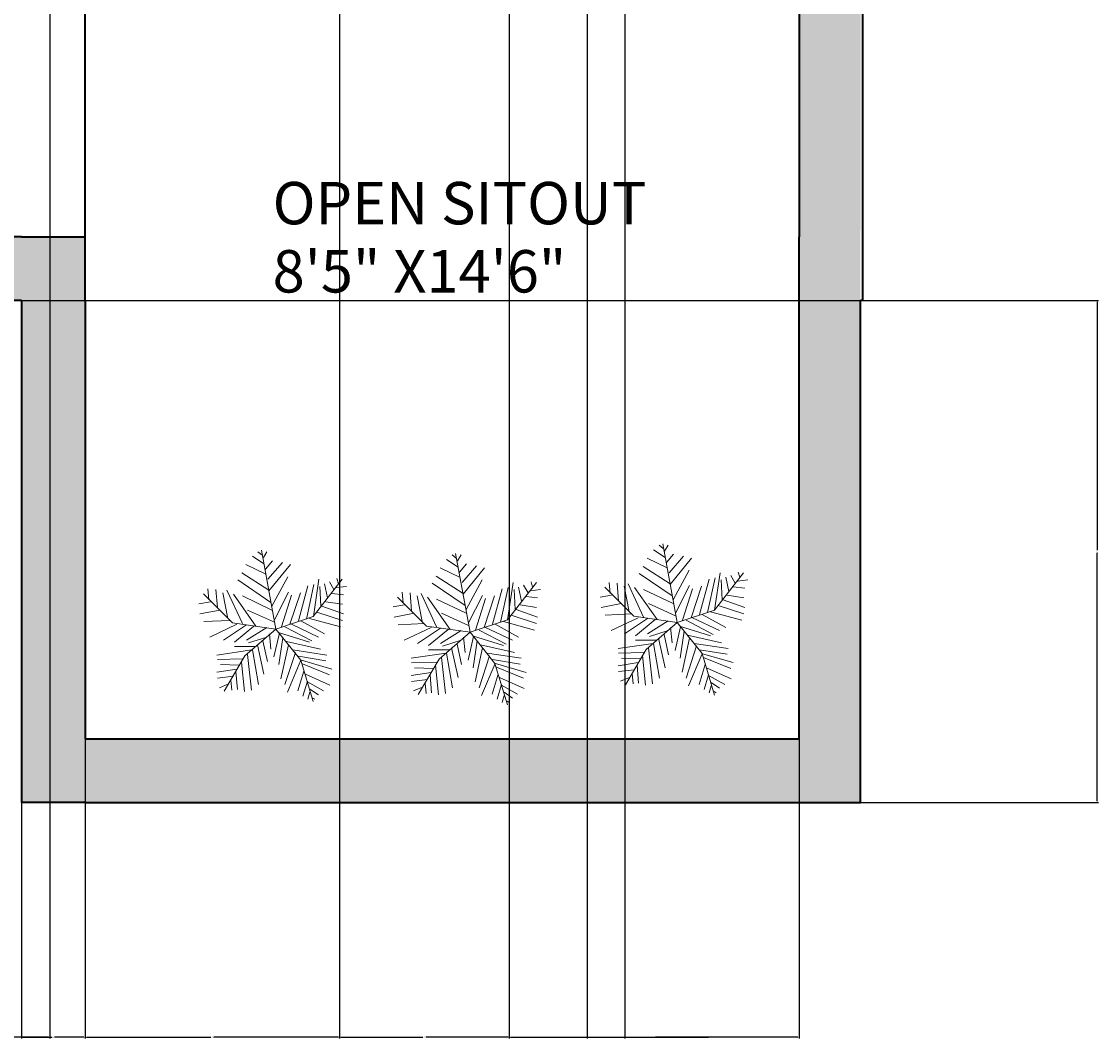
# Model space of a CAD drawing. Units: inches. Extents: x 2070 to 4408, y 1595 to 4269.
# Tile 5 of 20: x 2336 to 2489, y 1595 to 1739. Entities that reach past the tile are written whole.
import ezdxf

# ---------------------------------------------------------------- set-up
doc = ezdxf.new("R2010")
doc.units = ezdxf.units.IN
for name, color, linetype, lineweight in [('A-ANNO-DIMS', 2, 'Continuous', 18), ('A-AREA-IDEN', 7, 'Continuous', 18), ('A-WALL', 7, 'Continuous', 35), ('L-PLNT', 3, 'Continuous', 13)]:
    doc.layers.add(name, color=color, linetype=linetype, lineweight=lineweight)
doc.layers.add('A-WALL-PATT', color=18, linetype='Continuous', lineweight=13, true_color=0x000000)
doc.styles.get("Standard").update_dxf_attribs({"font": 'arial.ttf'})
doc.dimstyles.get("Standard").update_dxf_attribs({"dimtxt": 0.18, "dimasz": 0.18, "dimexe": 0.18, "dimexo": 0.0625, "dimgap": 0.09, "dimtad": 0, "dimtih": 1, "dimtoh": 1, "dimdec": 4, "dimzin": 0, "dimdsep": 46, "dimtxsty": 'Standard', "dimcen": 0.09, "dimadec": 0, "dimazin": 0, "dimtfac": 1, "dimtdec": 4, "dimtofl": 0, "dimtmove": 0, "dimatfit": 3, "dimfxl": 1, "dimtolj": 1, "dimtzin": 0, "dimarcsym": 0})

# ---------------------------------------------------------------- blocks, each defined once
blk = doc.blocks.new('Trees - Imperial')
for p, q in [((-10.186, 53.64), (-13.084, 55.962)), ((0, 0), (-10.5, 57)), ((-9.099, 51.782), (-6.563, 55.962)), ((-8.737, 47.138), (-17.069, 52.711)), ((-7.65, 43.423), (-2.578, 49.46)), ((-5.839, 35.992), (4.667, 48.067)), ((-5.114, 28.097), (-24.676, 40.636)), ((-7.288, 39.707), (-21.778, 46.673)), ((-5.114, 27.632), (10.463, 46.673)), ((-3.665, 19.273), (-27.574, 35.527)), ((-2.941, 16.486), (8.652, 37.85)), ((16.259, 5.805), (23.142, 31.348)), ((22.055, 7.198), (27.489, 32.277)), ((27, 9), (48, 36)), ((27.127, 9.056), (31.112, 35.992)), ((35.096, 32.741), (37.27, 22.524)), ((38.719, 34.134), (41.979, 28.561)), ((44.153, 36.456), (45.239, 32.741)), ((-31.5, 4.5), (-52.5, 25.5)), ((-48.585, 21.131), (-49.309, 29.026)), ((-43.513, 28.561), (-42.427, 15.558)), ((-38.442, 26.239), (-34.819, 7.663)), ((-35.544, 28.097), (-24.314, 3.947)), ((-14.533, 2.09), (-30.834, 25.31)), ((-24.314, 23.917), (-2.941, 13.7)), ((-1.129, 6.734), (9.014, 26.704)), ((3.942, 1.625), (11.187, 24.381)), ((10.101, 3.483), (17.708, 26.239)), ((31.836, 30.883), (32.561, 16.486)), ((40.53, 25.775), (48.862, 24.846)), ((43.791, 29.954), (51.036, 30.883)), ((-47.498, 19.737), (-55.83, 18.344)), ((33.285, 16.486), (48.862, 10.913)), ((36.183, 19.737), (48.137, 17.88)), ((-40.615, 13.7), (-55.105, 10.913)), ((-20.691, 13.7), (-1.129, 4.876)), ((0, 0), (27, 9)), ((29.662, 12.307), (48.137, 6.269)), ((-33.37, 6.269), (-52.207, 5.34)), ((-28.299, 3.483), (-47.86, -5.805)), ((-21.416, 3.018), (-38.079, -8.128)), ((0, 0), (-31.5, 4.5)), ((-15.982, 2.09), (-30.11, -9.521)), ((0, 0), (-22.5, -19.5)), ((-6.563, 1.161), (-21.416, -8.128)), ((0, 0), (18, -22.5)), ((6.478, 1.625), (26.04, -8.592)), ((11.187, 3.483), (30.749, -5.805)), ((18.07, 5.805), (35.096, -3.483)), ((24.229, 7.663), (46.688, 1.625)), ((-6.563, -5.805), (-19.967, -9.985)), ((-4.752, -3.483), (-3.665, -14.629)), ((2.493, -3.019), (-1.491, -20.202)), ((1.769, -2.555), (24.229, -9.521)), ((5.029, -6.27), (2.131, -25.775)), ((-17.431, -15.094), (-42.789, -18.809)), ((-15.257, -12.772), (-30.11, -12.772)), ((-17.069, -15.094), (-12.721, -40.172)), ((-13.446, -11.378), (-8.737, -32.741)), ((-9.461, -8.592), (-6.201, -23.453)), ((9.014, -11.378), (3.58, -35.992)), ((7.565, -9.056), (32.198, -14.629)), ((12.274, -15.094), (36.907, -18.809)), ((-24.314, -21.596), (-42.427, -22.06)), ((-22.5, -19.5), (-37.5, -45)), ((-20.691, -18.345), (-17.793, -44.352)), ((14.085, -16.951), (6.478, -40.172)), ((18.07, -22.524), (8.289, -45.745)), ((16.259, -19.738), (36.183, -22.989)), ((18, -22.5), (27, -52.5)), ((18.433, -22.524), (40.53, -29.026)), ((-28.299, -29.026), (-42.789, -31.348)), ((-26.849, -26.24), (-40.253, -25.775)), ((-29.023, -30.884), (-27.936, -43.887)), ((-25.038, -23.918), (-22.865, -45.281)), ((20.244, -30.419), (15.897, -44.816)), ((19.157, -25.311), (38.719, -33.206)), ((-30.834, -34.135), (-42.427, -35.528)), ((-32.646, -36.921), (-31.921, -44.352)), ((22.78, -37.85), (19.519, -48.532)), ((21.331, -32.741), (39.081, -40.636)), ((22.78, -38.314), (34.372, -44.816)), ((-34.457, -39.708), (-40.978, -42.494)), ((24.591, -45.745), (23.142, -50.854)), ((24.591, -43.423), (30.749, -47.603)), ((26.764, -49.925), (28.213, -50.854))]:
    blk.add_line(p, q)
blk = doc.blocks.new('*D26')
at = {"layer": 'A-ANNO-DIMS', "color": 0, "lineweight": -2, "transparency": 16777216}
for p, q in [((2336.26, 1699.4), (2488.56, 1699.4)), ((2488.38, 1699.22), (2488.38, 1664.08)), ((2488.38, 1628.58), (2488.38, 1663.72)), ((2454.95, 1628.4), (2488.56, 1628.4))]:
    blk.add_line(p, q, dxfattribs=at)
at = {"layer": 'A-ANNO-DIMS', "color": 0, "transparency": 16777216}
for points in [[(2488.35, 1699.22), (2488.41, 1699.22), (2488.38, 1699.4)], [(2488.35, 1628.58), (2488.41, 1628.58), (2488.38, 1628.4)]]:
    blk.add_solid(points, dxfattribs=at)
at = {"layer": 'Defpoints', "color": 0, "transparency": 16777216}
for p in [(2336.2, 1699.4), (2488.38, 1699.4), (2454.88, 1628.4)]:
    blk.add_point(p, dxfattribs=at)
at = {"layer": 'A-ANNO-DIMS', "color": 0, "transparency": 16777216, "insert": (2488.38, 1663.9), "char_height": 0.18, "attachment_point": 5}
blk.add_mtext('\\A1;71', dxfattribs=at)
blk = doc.blocks.new('*D27')
at = {"layer": 'A-ANNO-DIMS', "color": 0, "lineweight": -2, "transparency": 16777216}
for p, q in [((2345.2, 1637.34), (2345.2, 1595.04)), ((2336.2, 1628.34), (2336.2, 1595.04)), ((2336.38, 1595.22), (2340.55, 1595.22)), ((2345.02, 1595.22), (2340.85, 1595.22))]:
    blk.add_line(p, q, dxfattribs=at)
at = {"layer": 'A-ANNO-DIMS', "color": 0, "transparency": 16777216}
for points in [[(2336.38, 1595.25), (2336.38, 1595.19), (2336.2, 1595.22)], [(2345.02, 1595.25), (2345.02, 1595.19), (2345.2, 1595.22)]]:
    blk.add_solid(points, dxfattribs=at)
at = {"layer": 'Defpoints', "color": 0, "transparency": 16777216}
for p in [(2345.2, 1637.4), (2336.2, 1628.4), (2345.2, 1595.22)]:
    blk.add_point(p, dxfattribs=at)
at = {"layer": 'A-ANNO-DIMS', "color": 0, "transparency": 16777216, "insert": (2340.7, 1595.22), "char_height": 0.18, "attachment_point": 5}
blk.add_mtext('\\A1;9', dxfattribs=at)
blk = doc.blocks.new('*D30')
at = {"layer": 'A-ANNO-DIMS', "color": 0, "lineweight": -2, "transparency": 16777216}
for p, q in [((2416.2, 2080.34), (2416.2, 1595.04)), ((2446.2, 2080.34), (2446.2, 1595.04)), ((2416.38, 1595.22), (2430.98, 1595.22)), ((2446.02, 1595.22), (2431.41, 1595.22))]:
    blk.add_line(p, q, dxfattribs=at)
at = {"layer": 'A-ANNO-DIMS', "color": 0, "transparency": 16777216}
for points in [[(2416.38, 1595.25), (2416.38, 1595.19), (2416.2, 1595.22)], [(2446.02, 1595.25), (2446.02, 1595.19), (2446.2, 1595.22)]]:
    blk.add_solid(points, dxfattribs=at)
at = {"layer": 'Defpoints', "color": 0, "transparency": 16777216}
for p in [(2416.2, 2080.4), (2446.2, 2080.4), (2446.2, 1595.22)]:
    blk.add_point(p, dxfattribs=at)
at = {"layer": 'A-ANNO-DIMS', "color": 0, "transparency": 16777216, "insert": (2431.2, 1595.22), "char_height": 0.18, "attachment_point": 5}
blk.add_mtext('\\A1;30', dxfattribs=at)
blk = doc.blocks.new('*D32')
at = {"layer": 'A-ANNO-DIMS', "color": 0, "lineweight": -2, "transparency": 16777216}
for p, q in [((2245.2, 2230.58), (2245.2, 1595.04)), ((2340.2, 2230.58), (2340.2, 1595.04)), ((2245.38, 1595.22), (2292.48, 1595.22)), ((2340.02, 1595.22), (2292.92, 1595.22))]:
    blk.add_line(p, q, dxfattribs=at)
at = {"layer": 'A-ANNO-DIMS', "color": 0, "transparency": 16777216}
for points in [[(2245.38, 1595.25), (2245.38, 1595.19), (2245.2, 1595.22)], [(2340.02, 1595.25), (2340.02, 1595.19), (2340.2, 1595.22)]]:
    blk.add_solid(points, dxfattribs=at)
at = {"layer": 'Defpoints', "color": 0, "transparency": 16777216}
for p in [(2245.2, 2230.65), (2340.2, 2230.65), (2340.2, 1595.22)]:
    blk.add_point(p, dxfattribs=at)
at = {"layer": 'A-ANNO-DIMS', "color": 0, "transparency": 16777216, "insert": (2292.7, 1595.22), "char_height": 0.18, "attachment_point": 5}
blk.add_mtext('\\A1;95', dxfattribs=at)
blk = doc.blocks.new('*D34')
at = {"layer": 'A-ANNO-DIMS', "color": 0, "lineweight": -2, "transparency": 16777216}
for p, q in [((2421.53, 2212.34), (2421.53, 1595.04)), ((2446.2, 2212.34), (2446.2, 1595.04)), ((2421.71, 1595.22), (2433.4, 1595.22)), ((2446.02, 1595.22), (2434.33, 1595.22))]:
    blk.add_line(p, q, dxfattribs=at)
at = {"layer": 'A-ANNO-DIMS', "color": 0, "transparency": 16777216}
for points in [[(2421.71, 1595.25), (2421.71, 1595.19), (2421.53, 1595.22)], [(2446.02, 1595.25), (2446.02, 1595.19), (2446.2, 1595.22)]]:
    blk.add_solid(points, dxfattribs=at)
at = {"layer": 'Defpoints', "color": 0, "transparency": 16777216}
for p in [(2421.53, 2212.4), (2446.2, 2212.4), (2446.2, 1595.22)]:
    blk.add_point(p, dxfattribs=at)
at = {"layer": 'A-ANNO-DIMS', "color": 0, "transparency": 16777216, "insert": (2433.86, 1595.22), "char_height": 0.18, "attachment_point": 5}
blk.add_mtext('\\A1;24.663', dxfattribs=at)
blk = doc.blocks.new('*D36')
at = {"layer": 'A-ANNO-DIMS', "color": 0, "lineweight": -2, "transparency": 16777216}
for p, q in [((2345.2, 1792.34), (2345.2, 1595.04)), ((2381.2, 1792.34), (2381.2, 1595.04)), ((2345.38, 1595.22), (2362.98, 1595.22)), ((2381.02, 1595.22), (2363.41, 1595.22))]:
    blk.add_line(p, q, dxfattribs=at)
at = {"layer": 'A-ANNO-DIMS', "color": 0, "transparency": 16777216}
for points in [[(2345.38, 1595.25), (2345.38, 1595.19), (2345.2, 1595.22)], [(2381.02, 1595.25), (2381.02, 1595.19), (2381.2, 1595.22)]]:
    blk.add_solid(points, dxfattribs=at)
at = {"layer": 'Defpoints', "color": 0, "transparency": 16777216}
for p in [(2345.2, 1792.4), (2381.2, 1792.4), (2381.2, 1595.22)]:
    blk.add_point(p, dxfattribs=at)
at = {"layer": 'A-ANNO-DIMS', "color": 0, "transparency": 16777216, "insert": (2363.2, 1595.22), "char_height": 0.18, "attachment_point": 5}
blk.add_mtext('\\A1;36', dxfattribs=at)
blk = doc.blocks.new('*D37')
at = {"layer": 'A-ANNO-DIMS', "color": 0, "lineweight": -2, "transparency": 16777216}
for p, q in [((2381.2, 1792.34), (2381.2, 1595.04)), ((2405.2, 1792.34), (2405.2, 1595.04)), ((2381.38, 1595.22), (2392.98, 1595.22)), ((2405.02, 1595.22), (2393.42, 1595.22))]:
    blk.add_line(p, q, dxfattribs=at)
at = {"layer": 'A-ANNO-DIMS', "color": 0, "transparency": 16777216}
for points in [[(2381.38, 1595.25), (2381.38, 1595.19), (2381.2, 1595.22)], [(2405.02, 1595.25), (2405.02, 1595.19), (2405.2, 1595.22)]]:
    blk.add_solid(points, dxfattribs=at)
at = {"layer": 'Defpoints', "color": 0, "transparency": 16777216}
for p in [(2381.2, 1792.4), (2405.2, 1792.4), (2405.2, 1595.22)]:
    blk.add_point(p, dxfattribs=at)
at = {"layer": 'A-ANNO-DIMS', "color": 0, "transparency": 16777216, "insert": (2393.2, 1595.22), "char_height": 0.18, "attachment_point": 5}
blk.add_mtext('\\A1;24', dxfattribs=at)
blk = doc.blocks.new('*D38')
at = {"layer": 'A-ANNO-DIMS', "color": 0, "lineweight": -2, "transparency": 16777216}
for p, q in [((2405.2, 1792.34), (2405.2, 1595.04)), ((2446.2, 1792.34), (2446.2, 1595.04)), ((2405.38, 1595.22), (2425.49, 1595.22)), ((2446.02, 1595.22), (2425.9, 1595.22))]:
    blk.add_line(p, q, dxfattribs=at)
at = {"layer": 'A-ANNO-DIMS', "color": 0, "transparency": 16777216}
for points in [[(2405.38, 1595.25), (2405.38, 1595.19), (2405.2, 1595.22)], [(2446.02, 1595.25), (2446.02, 1595.19), (2446.2, 1595.22)]]:
    blk.add_solid(points, dxfattribs=at)
at = {"layer": 'Defpoints', "color": 0, "transparency": 16777216}
for p in [(2405.2, 1792.4), (2446.2, 1792.4), (2446.2, 1595.22)]:
    blk.add_point(p, dxfattribs=at)
at = {"layer": 'A-ANNO-DIMS', "color": 0, "transparency": 16777216, "insert": (2425.7, 1595.22), "char_height": 0.18, "attachment_point": 5}
blk.add_mtext('\\A1;41', dxfattribs=at)

msp = doc.modelspace()

# ---------------------------------------------------------------- hatches: boundary and pattern name
at = {"layer": 'A-WALL-PATT'}
h = msp.add_hatch(color=256, dxfattribs=at)
h.dxf.hatch_style = 1
h.paths.add_polyline_path([(2346.196, 2218.3995), (2346.196, 2282.3995), (2340.196, 2282.3995), (2340.196, 2212.3995), (2345.5866, 2212.3995), (2346.196, 2212.3995)], flags=0)
h.paths.add_polyline_path([(2245.196, 2282.3995), (2239.196, 2282.3995), (2239.196, 2186.3995), (2244.5866, 2186.3995), (2245.196, 2186.3995)], flags=0)
h.paths.add_polyline_path([(2340.196, 2230.6455), (2245.196, 2230.6455), (2245.196, 2224.6455), (2340.196, 2224.6455)], flags=0)
h.paths.add_polyline_path([(2245.196, 2150.3995), (2239.196, 2150.3995), (2164.4362, 2150.3995), (2164.4362, 2144.3995), (2239.196, 2144.3995), (2239.196, 2086.3995), (2239.196, 2067.2711), (2244.5866, 2067.2711), (2245.196, 2067.2711), (2245.196, 2144.3995)], flags=0)
h.paths.add_polyline_path([(2346.196, 2176.3995), (2340.196, 2176.3995), (2340.196, 2086.3995), (2346.196, 2086.3995), (2346.196, 2125.318)], flags=0)
h.paths.add_polyline_path([(2446.196, 2086.3995), (2346.196, 2086.3995), (2340.196, 2086.3995), (2340.196, 2080.3995), (2446.196, 2080.3995)], flags=0)
h.paths.add_polyline_path([(2455.196, 2291.3995), (2103.196, 2291.3995), (2103.196, 1699.3995), (2336.196, 1699.3995), (2336.196, 1628.3995), (2345.196, 1628.3995), (2446.196, 1628.3995), (2454.8846, 1628.3995), (2454.8846, 1699.3995)])
h.paths.add_polyline_path([(2446.196, 2282.3995), (2446.196, 2218.3995), (2446.196, 2212.3995), (2446.196, 2086.3995), (2446.196, 2080.3995), (2446.196, 1708.3995), (2446.196, 1637.3995), (2345.196, 1637.3995), (2345.196, 1699.3995), (2345.196, 1708.3995), (2336.196, 1708.3995), (2112.196, 1708.3995), (2112.196, 2282.3995), (2239.196, 2282.3995), (2245.196, 2282.3995), (2356.196, 2282.3995)], flags=16)
h.paths.add_polyline_path([(2245.196, 2150.3995), (2245.196, 2144.3995), (2245.196, 2067.2711), (2244.5866, 2067.2711), (2239.196, 2067.2711), (2239.196, 2065.6988), (2203.2929, 2065.6988, 0.40145271), (2239.196, 2031.3337), (2244.5866, 2031.3337), (2245.196, 2031.2711), (2245.196, 1924.1525), (2239.196, 1924.1525), (2239.196, 1922.5803), (2203.2929, 1922.5803, 0.40145271), (2239.196, 1888.2151), (2244.5866, 1888.2151), (2245.196, 1888.1525), (2245.196, 1748.3995), (2339.196, 1748.4621, -0.40145271), (2303.2929, 1782.8272), (2303.2585, 1782.8272), (2303.2585, 1784.3995), (2339.196, 1784.3995), (2339.196, 1877.2067), (2291.196, 1877.2067), (2291.196, 1883.2067), (2291.196, 1946.3995), (2291.196, 1952.3995), (2291.196, 2086.3995), (2297.196, 2086.3995), (2302.196, 2086.3995), (2302.196, 2081.0259), (2303.7633, 2081.0259), (2303.7633, 2080.3995), (2338.0148, 2080.3995, 0.00437129), (2338.0203, 2081.0259), (2338.0203, 2086.3995), (2340.196, 2086.3995), (2340.196, 2176.4621), (2345.5866, 2176.4621, 0.40145271), (2381.4896, 2210.8272), (2345.5866, 2210.8272), (2345.5866, 2212.3995), (2340.196, 2212.3995), (2340.196, 2224.6455), (2245.196, 2224.6455), (2245.196, 2186.3995), (2244.5866, 2186.3995), (2239.196, 2186.3995), (2239.196, 2184.8272), (2203.2929, 2184.8272, 0.40145271), (2239.196, 2150.4621), (2244.5866, 2150.4621)], flags=0)
h.paths.add_polyline_path([(2346.196, 2282.3995), (2346.196, 2218.3995), (2377.1813, 2218.3995), (2377.1813, 2212.3995), (2346.196, 2212.3995), (2345.5866, 2212.3995), (2340.196, 2212.3995), (2340.196, 2224.6455), (2245.196, 2224.6455), (2245.196, 2230.6455), (2245.196, 2282.3995), (2292.696, 2256.5225), (2340.196, 2282.3995)], flags=0)
h.paths.add_polyline_path([(2346.196, 2086.3995), (2340.196, 2086.3995), (2340.196, 2080.3995), (2446.196, 2080.3995), (2431.196, 2016.3995), (2446.196, 1952.3995), (2412.196, 1952.3995), (2412.196, 2080.3995), (2340.196, 2080.3995), (2340.196, 2086.3995), (2340.196, 2176.3995), (2346.196, 2176.3995), (2346.196, 2125.318)], flags=0)
h.paths.add_polyline_path([(2186.508, 2270.0471, -0.03755288), (2186.9712, 2269.8581), (2186.9164, 2270.112, -0.02759121)], flags=0)
h.paths.add_polyline_path([(2183.955, 2273.7766, 1), (2188.2945, 2273.7766, 1)], flags=0)
h.paths.add_polyline_path([(2142.5261, 2274.6158, -0.03707541), (2142.5672, 2275.1696), (2142.5672, 2276.826), (2119.8759, 2276.826), (2119.8759, 2263.0962), (2140.4332, 2263.0962), (2142.5672, 2263.0962), (2142.5672, 2274.0621, -0.03707541)], flags=0)
h.paths.add_polyline_path([(2209.8974, 2263.0962), (2209.8974, 2262.2079), (2190.8042, 2262.2079), (2190.8042, 2263.0962)], flags=0)
h.paths.add_polyline_path([(2210.6382, 2276.1833), (2210.6382, 2263.9844), (2190.2185, 2263.9844), (2190.2185, 2276.1833)], flags=0)
h.paths.add_polyline_path([(2188.4362, 2273.7766, -1), (2183.8133, 2273.7766, -1)], flags=0)
h.paths.add_polyline_path([(2245.196, 2150.3995), (2245.196, 2144.3995), (2245.196, 2067.2711), (2239.196, 2067.2711), (2239.196, 2080.3995), (2172.196, 2080.3995), (2172.196, 2000.3995), (2239.196, 2000.3995), (2239.196, 1940.3995), (2159.0187, 1940.3995), (2123.0187, 1940.3995), (2112.196, 1940.3995), (2112.196, 1946.3995), (2123.0187, 1946.3995), (2123.0187, 1982.2238), (2124.586, 1982.2238), (2124.586, 1982.1895, -0.40145271), (2158.8429, 1946.3995), (2159.0187, 1946.3995), (2239.196, 1946.3995), (2239.196, 1994.3995), (2112.196, 1994.3995), (2112.196, 2000.3995), (2139.196, 2040.3995), (2112.196, 2080.3995), (2112.196, 2086.3995), (2239.196, 2086.3995), (2239.196, 2144.3995), (2209.5809, 2144.3995), (2209.5809, 2136.3995), (2203.0809, 2136.3995), (2205.0809, 2130.3996, -0.70257121), (2199.081, 2116.3995, -0.70256205), (2193.0809, 2130.3994), (2195.0809, 2136.3995), (2192.0809, 2136.3995), (2192.0809, 2134.8995), (2189.0809, 2134.8995), (2189.0809, 2135.8995), (2191.0809, 2135.8995), (2191.0809, 2136.3995), (2188.5809, 2136.3995), (2188.5809, 2144.3995), (2164.2481, 2144.3995, -0.39385849), (2130.0035, 2109.5491), (2130.0035, 2109.5147), (2128.4362, 2109.5147), (2128.4362, 2144.3995), (2112.196, 2144.3995), (2112.196, 2150.3995), (2128.4362, 2150.3995), (2128.4362, 2150.7127), (2164.4362, 2150.7127), (2164.4362, 2150.3995), (2239.196, 2150.3995)], flags=0)
h.paths.add_polyline_path([(2188.2075, 2266.8735), (2188.2075, 2211.8632, -0.41421356), (2185.4833, 2209.1391), (2146.7995, 2209.1391, -0.41421356), (2144.0754, 2211.8632), (2144.0754, 2266.8735, -0.41421356), (2146.7995, 2269.5976), (2185.4833, 2269.5976, -0.41421356)], flags=0)
h.paths.add_polyline_path([(2185.0844, 2273.7766, -1), (2187.1651, 2273.7766, -1)], flags=0)
h.paths.add_polyline_path([(2182.0486, 2259.2932), (2168.0953, 2259.2932), (2168.0953, 2260.8424), (2163.7261, 2260.8424), (2163.7261, 2259.2932), (2149.7727, 2259.2932), (2149.7727, 2266.3352), (2163.7261, 2266.3352), (2163.7261, 2261.9839), (2168.0953, 2261.9839), (2168.0953, 2266.3352), (2182.0486, 2266.3352)], flags=0)
h.paths.add_polyline_path([(2148.2585, 2250.2051), (2153.0615, 2241.8861, 0.39807048)], flags=0)
h.paths.add_polyline_path([(2162.7572, 2247.2885), (2153.1461, 2241.7396), (2148.1083, 2250.4653), (2157.7194, 2256.0142)], flags=0)
h.paths.add_polyline_path([(2162.6726, 2247.4351, -0.39286196), (2157.8415, 2255.6313), (2157.6431, 2255.6313), (2157.8696, 2255.7541)], flags=0)
h.paths.add_polyline_path([(2164.2604, 2145.339), (2164.4362, 2144.3995), (2164.4362, 2150.3995), (2164.2604, 2150.7127)], flags=0)
h.paths.add_polyline_path([(2208.5809, 2142.6495), (2208.5809, 2138.3995, -0.41421356), (2207.8309, 2137.3995), (2190.5809, 2137.3995, -0.41421356), (2189.5809, 2138.1495), (2189.5809, 2142.3995, -0.41421356), (2190.3309, 2143.3995), (2207.5809, 2143.3995, -0.41421356)], flags=0)
h.paths.add_polyline_path([(2147.957, 2229.9119), (2154.7494, 2223.1195, 0.39807048)], flags=0)
h.paths.add_polyline_path([(2162.7165, 2230.8473), (2154.8691, 2222.9998), (2147.7446, 2230.1244), (2155.592, 2237.9718)], flags=0)
h.paths.add_polyline_path([(2162.5969, 2230.9669, -0.39807048), (2155.8044, 2237.7594)], flags=0)
h.paths.add_polyline_path([(2391.8776, 2049.9192), (2408.5766, 2049.9192), (2408.5766, 2033.2202), (2408.5766, 1983.123), (2408.5766, 1966.4239), (2391.8776, 1966.4239), (2391.8776, 1983.123), (2341.7804, 1983.123), (2341.7804, 2033.2202), (2391.8776, 2033.2202)], flags=0)
h.paths.add_polyline_path([(2144.1055, 2274.6158, 1), (2148.445, 2274.6158, 1)], flags=0)
h.paths.add_polyline_path([(2148.5867, 2274.6158, -1), (2143.9638, 2274.6158, -1)], flags=0)
h.paths.add_polyline_path([(2145.2349, 2274.6158, -1), (2147.3156, 2274.6158, -1)], flags=0)
edge = h.paths.add_edge_path(flags=0)
edge.add_ellipse((2400.5951, 2040.9436), major_axis=(-4.5109, 0), ratio=0.97544784, start_angle=180, end_angle=270, ccw=False)
edge.add_ellipse((2400.5951, 2040.9436), major_axis=(-4.5109, 0), ratio=0.97544784, start_angle=90, end_angle=180, ccw=False)
edge.add_ellipse((2400.5951, 2040.9436), major_axis=(-4.5109, 0), ratio=0.97544784, start_angle=0, end_angle=90, ccw=False)
edge.add_ellipse((2400.5951, 2040.9436), major_axis=(-4.5109, 0), ratio=0.97544784, start_angle=270, end_angle=360, ccw=False)
h.paths.add_polyline_path([(2199.0809, 2117.3995, -0.73452973), (2195.0809, 2130.3995), (2203.081, 2130.3995, -0.73453329)], flags=0)
h.paths.add_polyline_path([(2141.9147, 2276.0353), (2141.9147, 2263.9844), (2120.4685, 2263.9844), (2120.4685, 2276.0353)], flags=0)
h.paths.add_polyline_path([(2138.4481, 2273.4072), (2138.4481, 2266.7226), (2133.2801, 2266.7226), (2133.2801, 2273.4072)], flags=0)
h.paths.add_polyline_path([(2137.9691, 2272.9175), (2137.9691, 2272.204), (2135.4229, 2272.204), (2135.4229, 2271.6329), (2135.3221, 2270.1051), (2135.3221, 2269.0265), (2135.4229, 2268.6811), (2135.4229, 2267.2011), (2133.7212, 2267.2011), (2133.7212, 2268.6811), (2133.7983, 2269.9587), (2133.7983, 2271.2758), (2133.7212, 2271.6329), (2133.7212, 2273.0065), (2135.717, 2273.0065), (2135.717, 2272.9175)], flags=0)
h.paths.add_polyline_path([(2137.9215, 2271.8264), (2137.9215, 2271.3786), (2137.5182, 2271.3786), (2136.9355, 2271.3786), (2136.3529, 2271.3786), (2135.7703, 2271.3786), (2135.7703, 2271.8264), (2136.1736, 2271.8264), (2136.7562, 2271.8264), (2137.3389, 2271.8264)], flags=0)
h.paths.add_polyline_path([(2137.9215, 2271.692), (2137.5182, 2271.692), (2136.9355, 2271.513), (2137.3389, 2271.513)], flags=0)
h.paths.add_polyline_path([(2136.3529, 2271.692), (2135.7703, 2271.513), (2136.1736, 2271.513), (2136.7562, 2271.692)], flags=0)
h.paths.add_polyline_path([(2137.9215, 2271.513), (2137.5182, 2271.513), (2136.7562, 2271.747), (2136.7562, 2271.692), (2137.3389, 2271.692)], flags=0)
h.paths.add_polyline_path([(2137.8207, 2270.4664), (2137.8207, 2270.0971), (2137.8207, 2269.627), (2137.8207, 2269.1569), (2137.8207, 2268.6868), (2137.3837, 2268.6868), (2136.6442, 2268.6868), (2135.9271, 2268.6868), (2135.9271, 2269.0562), (2135.9271, 2269.5263), (2135.9271, 2269.9963), (2135.9271, 2270.4664), (2136.3641, 2270.4664), (2137.0812, 2270.4664)], flags=0)
h.paths.add_polyline_path([(2137.3837, 2269.627), (2137.8207, 2269.627), (2137.8207, 2269.5263), (2137.3837, 2269.5263), (2137.3837, 2269.1569), (2137.8207, 2269.1569), (2137.3837, 2269.0562), (2137.3837, 2268.6868), (2137.0812, 2268.6868), (2137.0812, 2269.0562), (2136.6442, 2269.0562), (2136.6442, 2268.6868), (2136.3641, 2268.6868), (2136.3641, 2269.0562), (2135.9271, 2269.0562), (2135.9271, 2269.1569), (2136.3641, 2269.1569), (2136.3641, 2269.5263), (2135.9271, 2269.5263), (2135.9271, 2269.627), (2136.3641, 2269.627), (2136.3641, 2269.9963), (2135.9271, 2269.9963), (2136.3641, 2270.0971), (2136.3641, 2270.4664), (2136.6442, 2270.4664), (2136.6442, 2270.0971), (2137.0812, 2270.0971), (2137.0812, 2270.4664), (2137.3837, 2270.4664), (2137.3837, 2270.0971), (2137.8207, 2270.0971), (2137.3837, 2269.9963)], flags=0)
h.paths.add_polyline_path([(2137.5182, 2271.8264), (2137.5182, 2271.692), (2137.3389, 2271.3786), (2137.3389, 2271.513)], flags=0)
h.paths.add_polyline_path([(2137.8179, 2267.8138), (2137.8179, 2267.6879), (2137.1876, 2267.6879), (2136.4733, 2267.6879), (2135.759, 2267.6879), (2135.759, 2267.8138), (2136.3893, 2267.8138), (2137.1036, 2267.8138)], flags=0)
h.paths.add_polyline_path([(2137.0812, 2269.9963), (2137.0812, 2269.627), (2137.0812, 2269.1569), (2136.6442, 2269.1569), (2136.6442, 2269.5263), (2136.6442, 2269.9963)], flags=0)
h.paths.add_polyline_path([(2136.3529, 2271.8264), (2136.3529, 2271.692), (2136.1736, 2271.3786), (2136.1736, 2271.513)], flags=0)
h.paths.add_polyline_path([(2136.4733, 2267.8138), (2136.4733, 2267.6879), (2136.3893, 2267.6879), (2136.3893, 2267.8138)], flags=0)
h.paths.add_polyline_path([(2407.9087, 2032.5522), (2407.9087, 1983.7909), (2359.81, 1983.7909, -0.00912788), (2359.0575, 1983.7909), (2342.4483, 1983.7909), (2342.4483, 2032.5522)], flags=0)
h.paths.add_polyline_path([(2389.1838, 2023.1358), (2353.7856, 2023.1358), (2353.7856, 1985.4867, -0.09210376), (2350.2788, 1988.655), (2350.2788, 2026.6426), (2389.1838, 2026.6426)], flags=0)
h.paths.add_polyline_path([(2352.6166, 2024.3048), (2351.4477, 2024.3048), (2351.4477, 2025.4737), (2352.6166, 2025.4737)], flags=0)
h.paths.add_polyline_path([(2399.6319, 2026.7589), (2404.3661, 2026.7589, -0.41421356), (2407.0379, 2024.087), (2407.0379, 2013.4908, -0.41421356), (2404.3661, 2010.819), (2399.6319, 2010.819, -0.41421356), (2396.96, 2013.4908), (2396.96, 2024.087, -0.41421356)], flags=0)
h.paths.add_polyline_path([(2399.6319, 2026.0909), (2404.3661, 2026.0909, -0.41421356), (2406.37, 2024.087), (2406.37, 2013.4908, -0.41421356), (2404.3661, 2011.487), (2399.6319, 2011.487, -0.41421356), (2397.628, 2013.4908), (2397.628, 2024.087, -0.41421356)], flags=0)
h.paths.add_polyline_path([(2399.6319, 2002.3217), (2404.3661, 2002.3217, -0.41421356), (2407.0379, 1999.6498), (2407.0379, 1989.0536, -0.41421356), (2404.3661, 1986.3818), (2399.6319, 1986.3818, -0.41421356), (2396.96, 1989.0536), (2396.96, 1999.6498, -0.41421356)], flags=0)
h.paths.add_polyline_path([(2399.6319, 2001.6537), (2404.3661, 2001.6537, -0.41421356), (2406.37, 1999.6498), (2406.37, 1989.0536, -0.41421356), (2404.3661, 1987.0497), (2399.6319, 1987.0497, -0.41421356), (2397.628, 1989.0536), (2397.628, 1999.6498, -0.41421356)], flags=0)
edge = h.paths.add_edge_path(flags=0)
edge.add_ellipse((2400.5951, 1975.3996), major_axis=(-4.5109, 0), ratio=0.97544784, start_angle=-180, end_angle=-90, ccw=False)
edge.add_ellipse((2400.5951, 1975.3996), major_axis=(-4.5109, 0), ratio=0.97544784, start_angle=90, end_angle=180, ccw=False)
edge.add_ellipse((2400.5951, 1975.3996), major_axis=(-4.5109, 0), ratio=0.97544784, start_angle=0, end_angle=90, ccw=False)
edge.add_ellipse((2400.5951, 1975.3996), major_axis=(-4.5109, 0), ratio=0.97544784, start_angle=-90, end_angle=0, ccw=False)
h.paths.add_polyline_path([(2345.196, 1910.3995), (2366.4386, 1910.3995), (2366.4386, 1925.4555), (2392.3856, 1925.4555), (2392.3856, 1933.5025), (2400.1399, 1925.4555), (2392.3856, 1919.8795), (2392.3856, 1925.4555), (2366.4386, 1925.4555), (2366.4386, 1910.3995), (2381.196, 1910.3995), (2405.196, 1910.3995), (2405.196, 1898.3995), (2446.196, 1898.3995), (2446.196, 1886.3995), (2405.196, 1886.3995), (2405.196, 1874.3995), (2446.196, 1874.3995), (2446.196, 1862.3995), (2405.196, 1862.3995), (2405.196, 1850.3995), (2446.196, 1850.3995), (2446.196, 1838.3995), (2405.196, 1838.3995), (2405.196, 1826.3995), (2446.196, 1826.3995), (2446.196, 1814.3995), (2405.196, 1814.3995), (2405.196, 1802.3995), (2446.196, 1802.3995), (2446.196, 1798.3995), (2446.196, 1792.3995), (2405.196, 1792.3995), (2405.196, 1910.3995), (2381.196, 1910.3995), (2381.196, 1792.3995), (2345.196, 1792.3995)], flags=0)
h.paths.add_polyline_path([(2333.0944, 1863.3993, -0.41421356), (2334.7225, 1861.7712), (2334.7225, 1859.329), (2335.2653, 1859.329, -0.41421356), (2337.4361, 1857.1582), (2337.4361, 1843.862, -0.41421356), (2335.2653, 1841.6911, -0.41421356), (2337.4361, 1839.5203), (2337.4361, 1827.5808, -0.41421356), (2335.2653, 1825.41, -0.41421356), (2337.4361, 1823.2392), (2337.4361, 1808.5862, -0.41421356), (2335.2653, 1806.4153), (2334.7225, 1806.4153), (2334.7225, 1803.9732, -0.41421356), (2333.0944, 1802.3451), (2317.356, 1802.3451), (2317.0846, 1802.3451, -0.41421356), (2315.7279, 1803.7018), (2315.7279, 1803.8646), (2313.8284, 1803.8646, -0.41421356), (2311.6576, 1806.0354), (2311.6576, 1823.2015, -0.39597602), (2313.6834, 1825.3765, -0.43384798), (2311.6576, 1827.2718), (2311.6576, 1839.761, -0.41421356), (2313.5571, 1841.6604), (2313.8284, 1841.6604), (2333.8159, 1841.6604, -0.04213623), (2334.1798, 1841.6911, -0.41421356), (2332.009, 1843.862), (2332.009, 1857.1582, -0.41421356), (2334.1798, 1859.329), (2317.356, 1859.329), (2317.0846, 1859.329, -0.41421356), (2315.7279, 1860.6858), (2315.7279, 1862.0426, -0.41421356), (2317.0846, 1863.3993), (2317.356, 1863.3993)], flags=0)
h.paths.add_polyline_path([(2208.8475, 1848.9818), (2208.8475, 1840.9741, -0.41421356), (2207.0458, 1839.1724), (2206.5453, 1839.1721), (2206.5453, 1838.7218, -0.40985861), (2204.7704, 1836.9203), (2183.7501, 1836.9203, -0.41858196), (2181.9216, 1838.7218), (2181.9216, 1839.1721), (2181.421, 1839.1724, -0.41421356), (2179.6193, 1840.9741), (2179.6193, 1848.6817, -0.44064415), (2185.1126, 1854.9874), (2203.3852, 1854.9874, -0.45707961)], flags=0)
h.paths.add_polyline_path([(2204.243, 1848.4815), (2204.243, 1848.4815, 0.41725335), (2202.2204, 1850.4833), (2186.2049, 1850.4833, 0.4111805), (2184.2237, 1848.4815), (2184.2237, 1848.4815, -0.4111807), (2186.2049, 1850.4833), (2202.2204, 1850.4833, -0.41725315)], flags=0)
h.paths.add_polyline_path([(2234.7177, 1830.228), (2234.7176, 1781.6047, -0.41421356), (2233.4381, 1780.3252), (2218.6064, 1780.3252, -0.41421356), (2217.8387, 1781.0929), (2217.8387, 1783.3961, -0.41421356), (2218.6064, 1784.1639), (2218.6065, 1796.9595, -0.41421356), (2219.886, 1798.239, -0.41421356), (2218.6065, 1799.5186), (2218.6065, 1812.3142, -0.41421356), (2219.8861, 1813.5938, -0.41421356), (2218.6065, 1814.8733), (2218.6065, 1827.6689, -0.41421356), (2217.8388, 1828.4367), (2217.8388, 1830.7399, -0.41421356), (2218.6065, 1831.5076), (2233.4382, 1831.5076, -0.41421356)], flags=0)
h.paths.add_polyline_path([(2230.6344, 1827.6689, -0.41421356), (2231.4021, 1826.9012), (2231.4021, 1784.9316, -0.41421356), (2230.6343, 1784.1639), (2221.1853, 1784.1639), (2221.1853, 1827.6689)], flags=0)
h.paths.add_polyline_path([(2222.7208, 1798.239), (2221.6971, 1798.239), (2221.6971, 1813.5938), (2222.7208, 1813.5938)], flags=0)
h.paths.add_polyline_path([(2206.5453, 1773.935), (2206.5453, 1773.4848), (2206.9457, 1773.4848), (2207.0458, 1773.4845, -0.41421356), (2208.8475, 1771.6827), (2208.8475, 1763.675, -0.44222432), (2203.6505, 1757.6695), (2185.3851, 1757.6695, -0.45508402), (2179.6193, 1763.9752), (2179.6193, 1771.6827, -0.41421356), (2181.421, 1773.4845), (2181.421, 1773.4848), (2181.9216, 1773.4848), (2181.9216, 1773.935, -0.40985861), (2183.6965, 1775.7366), (2204.7167, 1775.7366, -0.41858196)], flags=0)
h.paths.add_polyline_path([(2202.2619, 1762.1736), (2186.2464, 1762.1736, -0.41725315), (2184.2237, 1764.1754), (2184.2237, 1764.1754, 0.41725335), (2186.2464, 1762.1736), (2202.2619, 1762.1736, 0.4111805), (2204.243, 1764.1754), (2204.243, 1764.1754, -0.4111807)], flags=0)
h.paths.add_polyline_path([(2313.0034, 1713.1906), (2312.997, 1713.1697), (2313.0123, 1713.1612)], flags=0)
h.paths.add_polyline_path([(2305.7314, 1721.0488), (2305.6257, 1721.1994), (2305.4853, 1721.084)], flags=0)
h.paths.add_polyline_path([(2307.5562, 1726.1427), (2307.6186, 1726.1026), (2307.5737, 1726.0477), (2308.5692, 1720.6434), (2310.5345, 1721.2985), (2310.5721, 1721.411), (2310.6958, 1721.3523), (2313.8453, 1722.4021), (2314.9351, 1723.8033), (2314.9294, 1723.9165), (2315.0028, 1723.8903), (2313.874, 1722.4389), (2313.8697, 1722.4102), (2308.5692, 1720.6434), (2308.9864, 1720.122), (2309.0665, 1720.0971), (2309.053, 1720.0387), (2310.9235, 1717.7005), (2311.4182, 1717.6259), (2311.2918, 1717.2402), (2312.0655, 1716.2731), (2312.1081, 1716.2606), (2312.0969, 1716.2339), (2308.5692, 1720.6434), (2305.2249, 1717.745), (2305.232, 1717.704), (2305.1665, 1717.6944), (2308.5692, 1720.6434)], flags=0)
h.paths.add_polyline_path([(2288.2072, 1714.3431), (2288.2008, 1714.3222), (2288.216, 1714.3137)], flags=0)
h.paths.add_polyline_path([(2280.9352, 1722.2013), (2280.8295, 1722.3519), (2280.689, 1722.2365)], flags=0)
h.paths.add_polyline_path([(2282.76, 1727.2952), (2282.8224, 1727.2551), (2282.7775, 1727.2002), (2283.773, 1721.7959), (2285.7383, 1722.451), (2285.7759, 1722.5635), (2285.8995, 1722.5048), (2289.0491, 1723.5546), (2290.1389, 1724.9558), (2290.1332, 1725.069), (2290.2065, 1725.0428), (2289.0777, 1723.5915), (2289.0735, 1723.5628), (2283.773, 1721.7959), (2284.1901, 1721.2745), (2284.2703, 1721.2496), (2284.2567, 1721.1913), (2286.1273, 1718.8531), (2286.622, 1718.7785), (2286.4956, 1718.3927), (2287.2692, 1717.4256), (2287.3119, 1717.4131), (2287.3006, 1717.3864), (2283.773, 1721.7959), (2280.4286, 1718.8975), (2280.4357, 1718.8565), (2280.3703, 1718.8469), (2283.773, 1721.7959)], flags=0)
h.paths.add_polyline_path([(2302.0672, 1721.8694), (2301.8205, 1721.8572), (2301.7578, 1722.1787), (2299.415, 1724.5215), (2299.103, 1724.4694), (2299.0662, 1724.8703)], flags=0)
h.paths.add_polyline_path([(2264.5643, 1715.4956), (2264.5579, 1715.4747), (2264.5731, 1715.4662)], flags=0)
h.paths.add_polyline_path([(2257.2923, 1723.3538), (2257.1865, 1723.5044), (2257.0461, 1723.389)], flags=0)
h.paths.add_polyline_path([(2259.117, 1728.4477), (2259.1795, 1728.4077), (2259.1345, 1728.3527), (2260.13, 1722.9484), (2262.0954, 1723.6036), (2262.133, 1723.716), (2262.2566, 1723.6573), (2265.4061, 1724.7071), (2266.4959, 1726.1083), (2266.4902, 1726.2215), (2266.5636, 1726.1953), (2265.4348, 1724.744), (2265.4305, 1724.7153), (2260.13, 1722.9484), (2260.5472, 1722.427), (2260.6273, 1722.4022), (2260.6138, 1722.3438), (2262.4843, 1720.0056), (2262.979, 1719.931), (2262.8526, 1719.5452), (2263.6263, 1718.5781), (2263.6689, 1718.5656), (2263.6577, 1718.5389), (2260.13, 1722.9484), (2256.7857, 1720.05), (2256.7928, 1720.009), (2256.7273, 1719.9994), (2260.13, 1722.9484)], flags=0)
h.paths.add_polyline_path([(2277.2709, 1723.0219), (2277.0243, 1723.0097), (2276.9616, 1723.3312), (2274.6187, 1725.6741), (2274.3067, 1725.6219), (2274.27, 1726.0228)], flags=0)
h.paths.add_polyline_path([(2253.628, 1724.1744), (2253.3814, 1724.1622), (2253.3186, 1724.4838), (2250.9758, 1726.8266), (2250.6638, 1726.7744), (2250.627, 1727.1753)], flags=0)
h.paths.add_polyline_path([(2161.9194, 1715.4956), (2161.913, 1715.4747), (2161.9282, 1715.4662)], flags=0)
h.paths.add_polyline_path([(2154.6474, 1723.3538), (2154.5416, 1723.5044), (2154.4012, 1723.389)], flags=0)
h.paths.add_polyline_path([(2162.7899, 1724.744), (2162.7856, 1724.7153), (2157.4851, 1722.9484), (2157.9023, 1722.427), (2157.9824, 1722.4022), (2157.9689, 1722.3438), (2159.8394, 1720.0056), (2160.3341, 1719.931), (2160.2078, 1719.5452), (2160.9814, 1718.5781), (2161.024, 1718.5656), (2161.0128, 1718.5389), (2157.4851, 1722.9484), (2154.1408, 1720.05), (2154.1479, 1720.009), (2154.0824, 1719.9994), (2157.4851, 1722.9484), (2156.4721, 1728.4477), (2156.5346, 1728.4077), (2156.4896, 1728.3527), (2157.4851, 1722.9484), (2159.4505, 1723.6036), (2159.4881, 1723.716), (2159.6117, 1723.6573), (2162.7612, 1724.7071), (2163.851, 1726.1083), (2163.8453, 1726.2215), (2163.9187, 1726.1953)], flags=0)
h.paths.add_polyline_path([(2150.9831, 1724.1744), (2150.7365, 1724.1622), (2150.6738, 1724.4838), (2148.3309, 1726.8266), (2148.0189, 1726.7744), (2147.9822, 1727.1753)], flags=0)
h.paths.add_polyline_path([(2132.5099, 1716.6482), (2132.5035, 1716.6272), (2132.5187, 1716.6187)], flags=0)
h.paths.add_polyline_path([(2125.2379, 1724.5064), (2125.1322, 1724.6569), (2124.9917, 1724.5415)], flags=0)
h.paths.add_polyline_path([(2133.3804, 1725.8965), (2133.3762, 1725.8678), (2128.0757, 1724.101), (2128.4928, 1723.5795), (2128.5729, 1723.5547), (2128.5594, 1723.4963), (2130.43, 1721.1581), (2130.9246, 1721.0835), (2130.7983, 1720.6977), (2131.5719, 1719.7306), (2131.6146, 1719.7181), (2131.6033, 1719.6914), (2128.0757, 1724.101), (2124.7313, 1721.2025), (2124.7384, 1721.1615), (2124.6729, 1721.1519), (2128.0757, 1724.101), (2127.0626, 1729.6002), (2127.1251, 1729.5602), (2127.0801, 1729.5052), (2128.0757, 1724.101), (2130.041, 1724.7561), (2130.0786, 1724.8685), (2130.2022, 1724.8098), (2133.3517, 1725.8597), (2134.4415, 1727.2608), (2134.4358, 1727.3741), (2134.5092, 1727.3478)], flags=0)
h.paths.add_polyline_path([(2121.5736, 1725.3269), (2121.327, 1725.3148), (2121.2643, 1725.6363), (2118.9214, 1727.9791), (2118.6094, 1727.9269), (2118.5727, 1728.3279)], flags=0)
h.paths.add_polyline_path([(2433.3904, 1646.406), (2433.384, 1646.3851), (2433.3992, 1646.3766)], flags=0)
h.paths.add_polyline_path([(2426.1184, 1654.2642), (2426.0127, 1654.4148), (2425.8722, 1654.2994)], flags=0)
h.paths.add_polyline_path([(2427.9432, 1659.3581), (2428.0056, 1659.318), (2427.9606, 1659.2631), (2428.9562, 1653.8588), (2430.9215, 1654.514), (2430.9591, 1654.6264), (2431.0827, 1654.5677), (2434.2323, 1655.6175), (2435.322, 1657.0187), (2435.3163, 1657.1319), (2435.3897, 1657.1057), (2434.2609, 1655.6544), (2434.2567, 1655.6257), (2428.9562, 1653.8588), (2429.3733, 1653.3374), (2429.4534, 1653.3126), (2429.4399, 1653.2542), (2431.3105, 1650.916), (2431.8051, 1650.8414), (2431.6788, 1650.4556), (2432.4524, 1649.4885), (2432.4951, 1649.476), (2432.4838, 1649.4493), (2428.9562, 1653.8588), (2425.6118, 1650.9604), (2425.6189, 1650.9194), (2425.5535, 1650.9098), (2428.9562, 1653.8588)], flags=0)
h.paths.add_polyline_path([(2376.63, 1645.4912), (2376.6236, 1645.4703), (2376.6388, 1645.4617)], flags=0)
h.paths.add_polyline_path([(2369.358, 1653.3494), (2369.2523, 1653.5), (2369.1118, 1653.3845)], flags=0)
h.paths.add_polyline_path([(2371.1828, 1658.4432), (2371.2452, 1658.4032), (2371.2003, 1658.3482), (2372.1958, 1652.944), (2374.1611, 1653.5991), (2374.1987, 1653.7116), (2374.3224, 1653.6528), (2377.4719, 1654.7027), (2378.5617, 1656.1038), (2378.556, 1656.2171), (2378.6293, 1656.1908), (2377.5005, 1654.7395), (2377.4963, 1654.7108), (2372.1958, 1652.944), (2372.6129, 1652.4225), (2372.6931, 1652.3977), (2372.6795, 1652.3393), (2374.5501, 1650.0011), (2375.0448, 1649.9265), (2374.9184, 1649.5407), (2375.692, 1648.5737), (2375.7347, 1648.5611), (2375.7234, 1648.5344), (2372.1958, 1652.944), (2368.8514, 1650.0456), (2368.8586, 1650.0046), (2368.7931, 1649.995), (2372.1958, 1652.944)], flags=0)
h.paths.add_polyline_path([(2404.0947, 1645.0338), (2404.0883, 1645.0128), (2404.1035, 1645.0043)], flags=0)
h.paths.add_polyline_path([(2396.8227, 1652.892), (2396.717, 1653.0425), (2396.5765, 1652.9271)], flags=0)
h.paths.add_polyline_path([(2398.6475, 1657.9858), (2398.7099, 1657.9458), (2398.665, 1657.8908), (2399.6605, 1652.4866), (2401.6258, 1653.1417), (2401.6634, 1653.2541), (2401.7871, 1653.1954), (2404.9366, 1654.2453), (2406.0264, 1655.6464), (2406.0207, 1655.7596), (2406.094, 1655.7334), (2404.9652, 1654.2821), (2404.961, 1654.2534), (2399.6605, 1652.4866), (2400.0776, 1651.9651), (2400.1578, 1651.9403), (2400.1442, 1651.8819), (2402.0148, 1649.5437), (2402.5095, 1649.4691), (2402.3831, 1649.0833), (2403.1567, 1648.1162), (2403.1994, 1648.1037), (2403.1881, 1648.077), (2399.6605, 1652.4866), (2396.3162, 1649.5881), (2396.3233, 1649.5471), (2396.2578, 1649.5375), (2399.6605, 1652.4866)], flags=0)
h.paths.add_polyline_path([(2419.4532, 1658.0857), (2422.4541, 1655.0848), (2422.2075, 1655.0726), (2422.1448, 1655.3941), (2419.8019, 1657.737), (2419.4899, 1657.6848)], flags=0)
h.paths.add_polyline_path([(2390.1575, 1656.7135), (2393.1584, 1653.7125), (2392.9118, 1653.7004), (2392.8491, 1654.0219), (2390.5063, 1656.3647), (2390.1943, 1656.3125)], flags=0)
h.paths.add_polyline_path([(2362.6928, 1657.1709), (2365.6937, 1654.1699), (2365.4471, 1654.1578), (2365.3844, 1654.4793), (2363.0416, 1656.8221), (2362.7295, 1656.77)], flags=0)
h.paths.add_polyline_path([(2419.9523, 2037.8601), (2440.2872, 2037.8601), (2440.2872, 2047.1732), (2419.9523, 2047.1732)], flags=8)
h.paths.add_polyline_path([(2370.186, 1698.9005), (2413.6287, 1698.9005), (2413.6287, 1708.0908), (2370.186, 1708.0908)], flags=8)
h.paths.add_polyline_path([(2370.1656, 1708.5185), (2430.0857, 1708.5185), (2430.0857, 1717.8316), (2370.1656, 1717.8316)], flags=8)
h.paths.add_polyline_path([(2254.1469, 1788.1883), (2302.2471, 1788.1883), (2302.2471, 1797.3786), (2254.1469, 1797.3786)], flags=8)
h.paths.add_polyline_path([(2254.1264, 1797.8063), (2326.1448, 1797.8063), (2326.1448, 1807.1194), (2254.1264, 1807.1194)], flags=8)
h.paths.add_polyline_path([(2300.08, 1914.5069), (2338.861, 1914.5069), (2338.861, 1923.6972), (2300.08, 1923.6972)], flags=8)
h.paths.add_polyline_path([(2300.0595, 1924.1249), (2331.5882, 1924.1249), (2331.5882, 1933.438), (2300.0595, 1933.438)], flags=8)
h.paths.add_polyline_path([(2176.6905, 1716.4567), (2224.1441, 1716.4567), (2224.1441, 1725.647), (2176.6905, 1725.647)], flags=8)
h.paths.add_polyline_path([(2176.67, 1726.0747), (2245.9176, 1726.0747), (2245.9176, 1735.3878), (2176.67, 1735.3878)], flags=8)
h.paths.add_polyline_path([(2339.997, 2039.7696), (2388.1034, 2039.7696), (2388.1034, 2048.9661), (2339.997, 2048.9661)], flags=8)
h.paths.add_polyline_path([(2339.9776, 2049.3928), (2388.7204, 2049.3928), (2388.7204, 2058.7059), (2339.9776, 2058.7059)], flags=8)
h.paths.add_polyline_path([(2366.0063, 2161.3825), (2409.449, 2161.3825), (2409.449, 2170.5728), (2366.0063, 2170.5728)], flags=8)
h.paths.add_polyline_path([(2365.9868, 2171.0016), (2405.879, 2171.0016), (2405.879, 2180.3085), (2365.9868, 2180.3085)], flags=8)
h.paths.add_polyline_path([(2366.0102, 2247.0726), (2407.12, 2247.0726), (2407.12, 2256.263), (2366.0102, 2256.263)], flags=8)
h.paths.add_polyline_path([(2365.9897, 2256.6906), (2397.9686, 2256.6906), (2397.9686, 2266.0037), (2365.9897, 2266.0037)], flags=8)
h.paths.add_polyline_path([(2271.8465, 2102.7885), (2307.6541, 2102.7885), (2307.6541, 2111.9849), (2271.8465, 2111.9849)], flags=8)
h.paths.add_polyline_path([(2271.8281, 2112.4126), (2304.2673, 2112.4126), (2304.2673, 2121.7196), (2271.8281, 2121.7196)], flags=8)
h.paths.add_polyline_path([(2141.6408, 2187.5934), (2182.108, 2187.5934), (2182.108, 2196.7837), (2141.6408, 2196.7837)], flags=8)
h.paths.add_polyline_path([(2141.6203, 2197.2114), (2190.3631, 2197.2114), (2190.3631, 2206.5245), (2141.6203, 2206.5245)], flags=8)
h.paths.add_polyline_path([(2165.7271, 2103.039), (2211.5027, 2103.039), (2211.5027, 2112.2293), (2165.7271, 2112.2293)], flags=8)
h.paths.add_polyline_path([(2165.7077, 2112.658), (2185.1033, 2112.658), (2185.1033, 2121.965), (2165.7077, 2121.965)], flags=8)
h.paths.add_polyline_path([(2174.945, 2048.0789), (2211.3973, 2048.0789), (2211.3973, 2057.2693), (2174.945, 2057.2693)], flags=8)
h.paths.add_polyline_path([(2174.9256, 2057.698), (2194.3212, 2057.698), (2194.3212, 2067.0049), (2174.9256, 2067.0049)], flags=8)
h.paths.add_polyline_path([(2164.8305, 1965.8394), (2202.9649, 1965.8394), (2202.9649, 1975.0297), (2164.8305, 1975.0297)], flags=8)
h.paths.add_polyline_path([(2164.8111, 1975.4584), (2184.2067, 1975.4584), (2184.2067, 1984.7654), (2164.8111, 1984.7654)], flags=8)
h.paths.add_polyline_path([(2133.0392, 1862.086), (2173.5065, 1862.086), (2173.5065, 1871.2763), (2133.0392, 1871.2763)], flags=8)
h.paths.add_polyline_path([(2133.0709, 1871.8585), (2157.0382, 1871.8585), (2157.0382, 1880.8585), (2133.0709, 1880.8585)], flags=8)
h.paths.add_polyline_path([(2406.4423, 1923.5541), (2418.8209, 1923.5541), (2418.8209, 1932.7199), (2406.4423, 1932.7199)], flags=8)

# ---------------------------------------------------------------- linework, layer by layer
at = {"layer": 'A-WALL'}
for p, q in [((2345.196, 1708.3995), (2345.196, 1742.3995)), ((2336.196, 1708.3995), (2345.196, 1708.3995)), ((2345.196, 1699.3995), (2345.196, 1708.3995)), ((2446.196, 1637.3995), (2446.196, 1708.3995)), ((2336.196, 1699.3995), (2336.196, 1628.3995)), ((2345.196, 1699.3995), (2345.196, 1637.3995)), ((2454.8846, 1628.3995), (2454.8846, 1699.3995)), ((2345.196, 1637.3995), (2446.196, 1637.3995)), ((2345.196, 1628.3995), (2336.196, 1628.3995)), ((2345.196, 1628.3995), (2446.196, 1628.3995)), ((2446.196, 1628.3995), (2454.8846, 1628.3995))]:
    msp.add_line(p, q, dxfattribs=at)
for points in [[(2336.196, 1699.3995), (2103.196, 1699.3995), (2103.196, 2291.3995), (2455.196, 2291.3995), (2455.196, 1699.3995), (2454.8846, 1699.3995)], [(2336.196, 1708.3995), (2112.196, 1708.3995), (2112.196, 2282.3995), (2446.196, 2282.3995), (2446.196, 2218.3995)], [(2446.196, 2212.3995), (2446.196, 1708.3995)]]:
    msp.add_lwpolyline(points, dxfattribs=at)

# ---------------------------------------------------------------- block references
at = {"layer": 'L-PLNT', "xscale": 0.1954109391421404, "yscale": 0.1954109391421404, "zscale": 0.1954109391421404}
for p in [(2372.1958, 1652.944), (2428.9562, 1653.8588), (2399.6605, 1652.4866)]:
    msp.add_blockref('Trees - Imperial', p, dxfattribs=at)

# ---------------------------------------------------------------- texts
at = {"layer": 'A-AREA-IDEN'}
for s, p in [('OPEN SITOUT', (2371.7177, 1710.173)), ('8\'5" X14\'6"', (2371.7177, 1700.5345))]:
    msp.add_text(s, height=6, dxfattribs=at).set_placement(p)

# ---------------------------------------------------------------- dimensions: what is measured, and where the dimension line sits
at = {"layer": 'A-ANNO-DIMS'}
for base, p1, p2, override, picture, middle in [((2340.196, 1595.2195), (2245.196, 2230.6455), (2340.196, 2230.6455), {"dimdec": 0, "dimlfac": 1, "dimrnd": 0, "dimzin": 0, "dimdsep": 46, "dimlunit": 2}, '*D32', (2292.696, 1595.2195)), ((2446.196, 1595.2195), (2421.5333, 2212.3995), (2446.196, 2212.3995), {"dimdec": 3, "dimlfac": 1, "dimrnd": 0, "dimzin": 0, "dimdsep": 46, "dimlunit": 2}, '*D34', (2433.8646, 1595.2195)), ((2446.196, 1595.2195), (2416.196, 2080.3995), (2446.196, 2080.3995), {"dimdec": 0, "dimlfac": 1, "dimrnd": 0, "dimzin": 0, "dimdsep": 46, "dimlunit": 2}, '*D30', (2431.196, 1595.2195)), ((2381.196, 1595.2195), (2345.196, 1792.3995), (2381.196, 1792.3995), {"dimdec": 0, "dimlfac": 1, "dimrnd": 0, "dimzin": 0, "dimdsep": 46, "dimlunit": 2}, '*D36', (2363.196, 1595.2195)), ((2405.196, 1595.2195), (2381.196, 1792.3995), (2405.196, 1792.3995), {"dimdec": 0, "dimlfac": 1, "dimrnd": 0, "dimzin": 0, "dimdsep": 46, "dimlunit": 2}, '*D37', (2393.196, 1595.2195)), ((2446.196, 1595.2195), (2405.196, 1792.3995), (2446.196, 1792.3995), {"dimdec": 0, "dimlfac": 1, "dimrnd": 0, "dimzin": 0, "dimdsep": 46, "dimlunit": 2}, '*D38', (2425.696, 1595.2195)), ((2345.196, 1595.2195), (2336.196, 1628.3995), (2345.196, 1637.3995), {"dimdec": 0, "dimlfac": 1, "dimrnd": 0, "dimzin": 0, "dimdsep": 46, "dimlunit": 2}, '*D27', (2340.696, 1595.2195))]:
    dim = msp.add_linear_dim(base=base, p1=p1, p2=p2, dimstyle='Standard', override=override, dxfattribs=at)
    dim.commit()
    dim.dimension.update_dxf_attribs({"geometry": picture, "text_midpoint": middle})
dim = msp.add_linear_dim(base=(2488.376, 1699.3995), p1=(2454.8846, 1628.3995), p2=(2336.196, 1699.3995), angle=90, dimstyle='Standard', override={"dimdec": 0, "dimlfac": 1, "dimrnd": 0, "dimzin": 0, "dimdsep": 46, "dimlunit": 2}, dxfattribs=at)
dim.commit()
dim.dimension.update_dxf_attribs({"geometry": '*D26', "text_midpoint": (2488.376, 1663.8995)})

doc.saveas('drawing.dxf')
